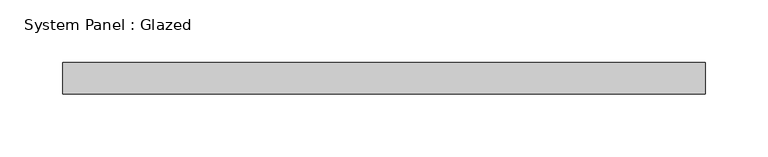
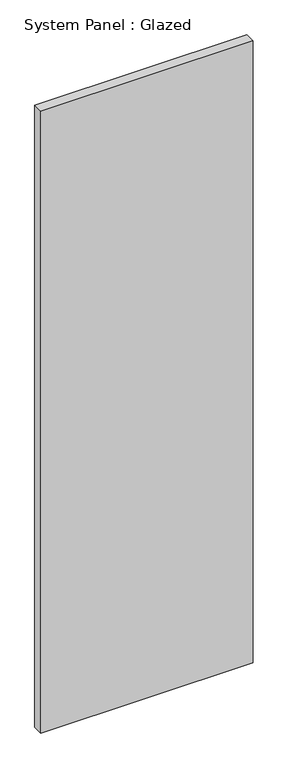
"""IFC4 building model written with IfcOpenShell, lengths in millimetres: plate geometry, System Panel : Glazed."""

from ifc_helpers import new_model, si_unit, origin, origin_with_axes, place, context, project, spatial, polyline, outline, extrude, source, transform, mapped, element, save


def system_panel_glazed_f636780f(model_context):
    return source(origin(), model_context, "Body", "SweptSolid", [
        extrude(outline(polyline([(257.175, 19.05), (-257.175, 19.05), (-257.175, 44.45), (257.175, 44.45), (257.175, 19.05)])), origin_with_axes(), (0.0, 0.0, 1.0), 1593.9224616),
    ])


if __name__ == "__main__":
    model = new_model("IFC4")
    model_context = context("Model", 3, world=origin())
    ifc_project = project(units=[si_unit("LENGTHUNIT", "METRE", prefix="MILLI")], contexts=[model_context])
    site = spatial("IfcSite", under=ifc_project)
    building = spatial("IfcBuilding", under=site)
    placement = place(None, origin())
    system_panel_glazed_shape = system_panel_glazed_f636780f(model_context)
    element("IfcPlate", 1, ObjectType="System Panel : Glazed", at=placement, inside=building, context=model_context, shape_type="MappedRepresentation", body=[
        mapped(system_panel_glazed_shape, transform((0.0, 0.0, 0.0), x_axis=(1.0, 0.0, 0.0), y_axis=(0.0, 1.0, 0.0), z_axis=(0.0, 0.0, 1.0))),
    ])
    save(model, "model.ifc")

# Revit data of these elements
# Type "System Panel : Glazed"
#   Construction Type Id = "GSP4R"
#   Analytic Construction = "1/8 in Pilkington single glazing"
#   Visual Light Transmittance = 0.9
#   Solar Heat Gain Coefficient = 0.86
#   Heat Transfer Coefficient (U) = 1.18115 BTU/(h·ft²·°F)
#   Define Thermal Properties by = 1
# Element 1 (IfcPlate, "System Panel : Glazed")
#   Materials on its faces: "Glass"
# Materials
#   "Glass": class "Glass", colour RGB 0 128 192, transparency 0.75, Description = "Soda Lime Glass", Cost = 0
